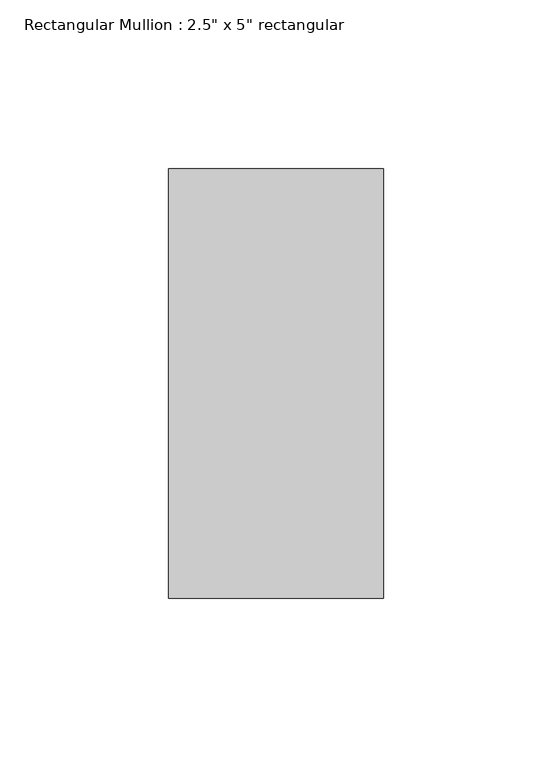
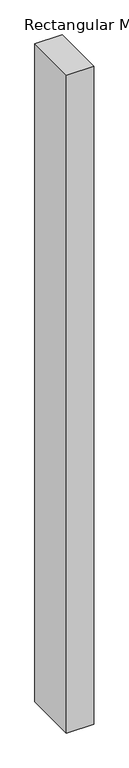
"""IFC4 building model written with IfcOpenShell, lengths in millimetres: member geometry."""

from ifc_helpers import new_model, si_unit, frame, origin, place, context, project, spatial, polyline, outline, extrude, source, transform, mapped, element, save


def member_037f74fd(model_context):
    return source(origin(), model_context, "Body", "SweptSolid", [
        extrude(outline(polyline([(31.75, 63.5), (31.75, -63.5), (-31.75, -63.5), (-31.75, 63.5), (31.75, 63.5)])), frame((0.0, 0.0, -1618.023499), z_axis=(0.0, 0.0, 1.0), x_axis=(1.0, 0.0, 0.0)), (0.0, 0.0, 1.0), 1618.023499),
    ])


if __name__ == "__main__":
    model = new_model("IFC4")
    model_context = context("Model", 3, world=origin())
    ifc_project = project(units=[si_unit("LENGTHUNIT", "METRE", prefix="MILLI")], contexts=[model_context])
    site = spatial("IfcSite", under=ifc_project)
    building = spatial("IfcBuilding", under=site)
    placement = place(None, origin())
    member_shape = member_037f74fd(model_context)
    element("IfcMember", 1, ObjectType="Rectangular Mullion : 2.5\" x 5\" rectangular", at=placement, inside=building, context=model_context, shape_type="MappedRepresentation", body=[
        mapped(member_shape, transform((0.0, 0.0, 0.0), x_axis=(1.0, 0.0, 0.0), y_axis=(0.0, 1.0, 0.0), z_axis=(0.0, 0.0, 1.0))),
    ])
    save(model, "model.ifc")

# Revit data of these elements
# Type "Rectangular Mullion : 2.5\" x 5\" rectangular"
#   built-in parameter 1007304 = 0.416667 (stored number, unit not read)
#   built-in parameter 1007301 = 0.104167 (stored number, unit not read)
#   built-in parameter 1007300 = 0.104167 (stored number, unit not read)
# Element 1 (IfcMember, "Rectangular Mullion : 2.5\" x 5\" rectangular")
#   Materials on its faces: "Aluminum"
# Materials
#   "Aluminum": class "Metal", colour RGB 247 247 247, transparency 0, Description = "Aluminum 6061", Cost = 0
